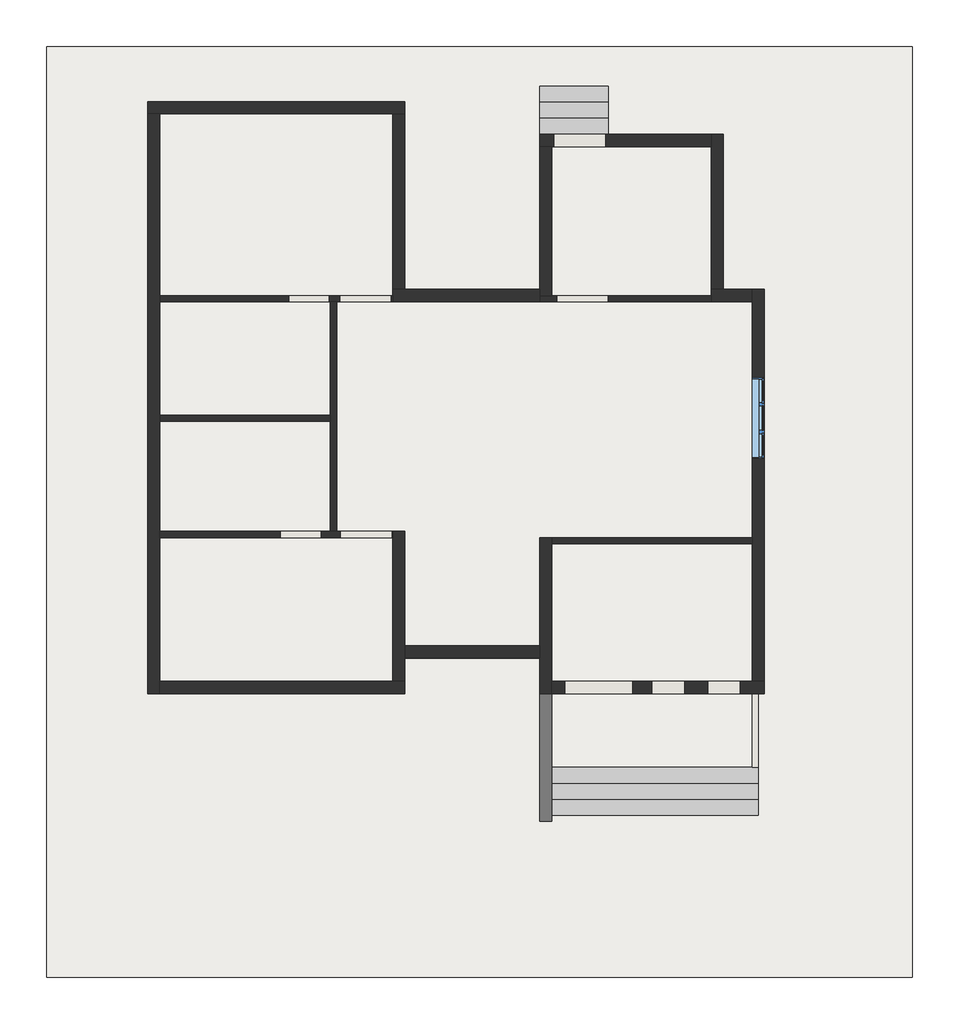
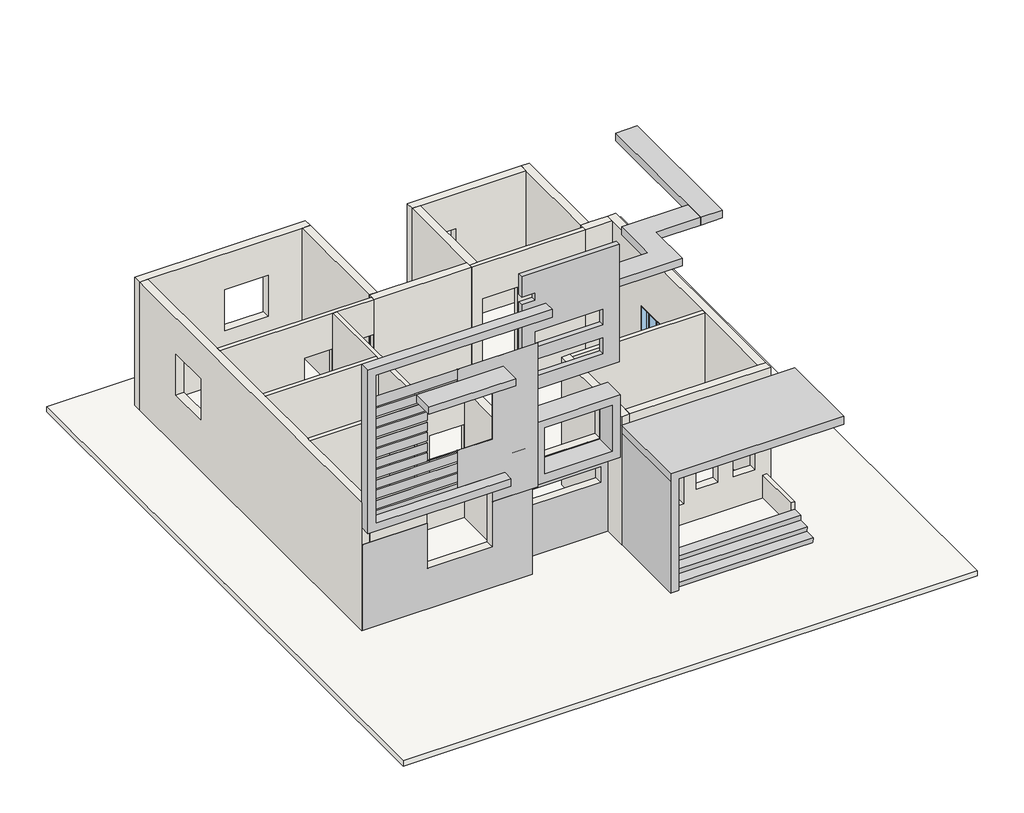
# One storey: 21 walls, 2 stair flights, 1 proxy, 1 slab, 1 window.
"""IFC4 building model written with IfcOpenShell, lengths in millimetres."""

from ifc_helpers import new_model, si_unit, frame, origin, origin_with_axes, place, context, project, spatial, polyline, outline, extrude, faceted_brep, transform, mapped, element, save
from components import generic_models_1_generic_models_1_ca1a1a43, window_casement_triple_middle_transom_5_x4_de6e65d4

model = new_model("IFC4")

# Units and contexts
model_context = context("Model", 3, world=origin())
ifc_project = project(units=[si_unit("LENGTHUNIT", "METRE", prefix="MILLI")], contexts=[model_context])

# Site, building, storey
site = spatial("IfcSite", under=ifc_project)
building = spatial("IfcBuilding", under=site)
storey = spatial("IfcBuildingStorey", under=building, Elevation=0.0)

# Proxy
placement = place(None, origin())
generic_models_1_generic_models_1_shape = generic_models_1_generic_models_1_ca1a1a43(model_context)
element("IfcBuildingElementProxy", 1, Name="Generic Models 1 : Generic Models 1", ObjectType="Generic Models 1 : Generic Models 1", at=placement, inside=storey, context=model_context, shape_type="MappedRepresentation", body=[
    mapped(generic_models_1_generic_models_1_shape, transform((0.0, 0.0, 0.0), x_axis=(1.0, 0.0, 0.0), y_axis=(0.0, 1.0, 0.0), z_axis=(0.0, 0.0, 1.0))),
])

# Slab
element("IfcSlab", 2, ObjectType="site floor", at=placement, inside=storey, context=model_context, shape_type="SweptSolid", body=[
    extrude(outline(polyline([(6700.8181677, 11356.791643), (6700.8181677, -6016.808357), (-9453.5818323, -6016.808357), (-9453.5818323, 11356.791643), (6700.8181677, 11356.791643)])), frame((0.0, 0.0, -152.4), z_axis=(0.0, 0.0, 1.0), x_axis=(1.0, 0.0, 0.0)), (0.0, 0.0, 1.0), 152.4),
])

# Stair flights
element("IfcStairFlight", 3, ObjectType="00 steps", at=placement, inside=storey, context=model_context, shape_type="Brep", body=[
    faceted_brep([(3826.8250448, -2992.8214711, 152.4), (-21.2749552, -2992.8214711, 152.4), (-21.2749552, -2973.7714711, 0.0), (3826.8250448, -2973.7714711, 0.0), (3826.8250448, -2673.7339711, 152.4), (-21.2749552, -2673.7339711, 152.4), (-21.2749552, -2673.7339711, 0.0), (3826.8250448, -2673.7339711, 0.0), (-21.2749552, -2692.7839711, 304.8), (3826.8250448, -2692.7839711, 304.8), (3826.8250448, -2373.7339711, 304.8), (-21.2749552, -2373.7339711, 304.8), (-21.2749552, -2373.7339711, 0.0), (3826.8250448, -2373.7339711, 0.0), (-21.2749552, -2092.7839711, 0.0), (3826.8250448, -2092.7839711, 0.0), (-21.2749552, -2392.7839711, 457.2), (3826.8250448, -2392.7839711, 457.2), (3826.8250448, -2092.7839711, 457.2), (-21.2749552, -2092.7839711, 457.2)], [[[0, 1, 2, 3]], [[1, 0, 4, 5]], [[1, 5, 6, 2]], [[4, 0, 3, 7]], [[8, 9, 10, 11]], [[6, 5, 8, 11, 12]], [[4, 7, 13, 10, 9]], [[5, 4, 9, 8]], [[2, 6, 12, 14, 15, 13, 7, 3]], [[16, 17, 18, 19]], [[12, 11, 16, 19, 14]], [[10, 13, 15, 18, 17]], [[19, 18, 15, 14]], [[11, 10, 17, 16]]]),
])
element("IfcStairFlight", 4, ObjectType="00 steps", at=placement, inside=storey, context=model_context, shape_type="Brep", body=[
    faceted_brep([(-249.8749552, 10618.0535289, 152.4), (1032.8250448, 10618.0535289, 152.4), (1032.8250448, 10599.0035289, 0.0), (-249.8749552, 10599.0035289, 0.0), (-249.8749552, 10298.9660289, 152.4), (1032.8250448, 10298.9660289, 152.4), (1032.8250448, 10298.9660289, 0.0), (-249.8749552, 10298.9660289, 0.0), (1032.8250448, 10318.0160289, 304.8), (-249.8749552, 10318.0160289, 304.8), (-249.8749552, 9998.9660289, 304.8), (1032.8250448, 9998.9660289, 304.8), (1032.8250448, 9998.9660289, 0.0), (-249.8749552, 9998.9660289, 0.0), (1032.8250448, 9718.0160289, 0.0), (-249.8749552, 9718.0160289, 0.0), (1032.8250448, 10018.0160289, 457.2), (-249.8749552, 10018.0160289, 457.2), (-249.8749552, 9718.0160289, 457.2), (1032.8250448, 9718.0160289, 457.2)], [[[0, 1, 2, 3]], [[1, 0, 4, 5]], [[1, 5, 6, 2]], [[4, 0, 3, 7]], [[8, 9, 10, 11]], [[6, 5, 8, 11, 12]], [[4, 7, 13, 10, 9]], [[5, 4, 9, 8]], [[2, 6, 12, 14, 15, 13, 7, 3]], [[16, 17, 18, 19]], [[12, 11, 16, 19, 14]], [[10, 13, 15, 18, 17]], [[19, 18, 15, 14]], [[11, 10, 17, 16]]]),
])

# Walls
element("IfcWall", 5, ObjectType="4.5\" wall", at=placement, inside=storey, context=model_context, shape_type="Brep", body=[
    faceted_brep([(-2993.0749552, 6708.1160289, 0.0), (-7336.4749552, 6708.1160289, 0.0), (-7336.4749552, 6708.1160289, 3810.0), (-2993.0749552, 6708.1160289, 3810.0), (-3018.4749552, 6708.1160289, 609.6), (-3018.4749552, 6708.1160289, 2768.6), (-3983.6749552, 6708.1160289, 2768.6), (-3983.6749552, 6708.1160289, 609.6), (-4936.1749552, 6708.1160289, 609.6), (-4174.1749552, 6708.1160289, 609.6), (-4174.1749552, 6708.1160289, 2743.2), (-4936.1749552, 6708.1160289, 2743.2), (-7336.4749552, 6593.8160289, 0.0), (-4155.1249552, 6593.8160289, 0.0), (-4040.8249552, 6593.8160289, 0.0), (-2993.0749552, 6593.8160289, 0.0), (-2993.0749552, 6593.8160289, 3810.0), (-4040.8249552, 6593.8160289, 3810.0), (-4155.1249552, 6593.8160289, 3810.0), (-7336.4749552, 6593.8160289, 3810.0), (-3018.4749552, 6593.8160289, 2768.6), (-3018.4749552, 6593.8160289, 609.6), (-3983.6749552, 6593.8160289, 609.6), (-3983.6749552, 6593.8160289, 2768.6), (-4936.1749552, 6593.8160289, 609.6), (-4936.1749552, 6593.8160289, 2743.2), (-4174.1749552, 6593.8160289, 2743.2), (-4174.1749552, 6593.8160289, 609.6)], [[[0, 1, 2, 3], [4, 5, 6, 7], [8, 9, 10, 11]], [[12, 13, 14, 15, 16, 17, 18, 19], [20, 21, 22, 23], [24, 25, 26, 27]], [[1, 0, 15, 14, 13, 12]], [[3, 2, 19, 18, 17, 16]], [[0, 3, 16, 15]], [[2, 1, 12, 19]], [[4, 21, 20, 5]], [[5, 20, 23, 6]], [[6, 23, 22, 7]], [[21, 4, 7, 22]], [[9, 8, 24, 27]], [[10, 9, 27, 26]], [[11, 10, 26, 25]], [[8, 11, 25, 24]]]),
])
element("IfcWall", 6, ObjectType="4.5\" wall", at=placement, inside=storey, context=model_context, shape_type="Brep", body=[
    faceted_brep([(-4155.1249552, 6593.8160289, 0.0), (-4155.1249552, 4479.2660289, 0.0), (-4155.1249552, 4364.9660289, 0.0), (-4155.1249552, 2307.5660289, 0.0), (-4155.1249552, 2307.5660289, 3810.0), (-4155.1249552, 4364.9660289, 3810.0), (-4155.1249552, 4479.2660289, 3810.0), (-4155.1249552, 6593.8160289, 3810.0), (-4040.8249552, 6593.8160289, 0.0), (-4040.8249552, 6593.8160289, 3810.0), (-4040.8249552, 2307.5660289, 3810.0), (-4040.8249552, 2307.5660289, 0.0)], [[[0, 1, 2, 3, 4, 5, 6, 7]], [[8, 9, 10, 11]], [[3, 2, 1, 0, 8, 11]], [[7, 6, 5, 4, 10, 9]], [[0, 7, 9, 8]], [[4, 3, 11, 10]]]),
])
element("IfcWall", 7, ObjectType="4.5\" wall", at=placement, inside=storey, context=model_context, shape_type="Brep", body=[
    faceted_brep([(-2993.0749552, 2307.5660289, 0.0), (-4040.8249552, 2307.5660289, 0.0), (-4155.1249552, 2307.5660289, 0.0), (-7336.4749552, 2307.5660289, 0.0), (-7336.4749552, 2307.5660289, 3810.0), (-4155.1249552, 2307.5660289, 3810.0), (-4040.8249552, 2307.5660289, 3810.0), (-2993.0749552, 2307.5660289, 3810.0), (-3005.7749552, 2307.5660289, 609.6), (-3005.7749552, 2307.5660289, 2768.6), (-3970.9749552, 2307.5660289, 2768.6), (-3970.9749552, 2307.5660289, 609.6), (-5088.5749552, 2307.5660289, 609.6), (-4326.5749552, 2307.5660289, 609.6), (-4326.5749552, 2307.5660289, 2743.2), (-5088.5749552, 2307.5660289, 2743.2), (-7336.4749552, 2193.2660289, 0.0), (-2993.0749552, 2193.2660289, 0.0), (-2993.0749552, 2193.2660289, 3810.0), (-7336.4749552, 2193.2660289, 3810.0), (-3005.7749552, 2193.2660289, 2768.6), (-3005.7749552, 2193.2660289, 609.6), (-3970.9749552, 2193.2660289, 609.6), (-3970.9749552, 2193.2660289, 2768.6), (-5088.5749552, 2193.2660289, 609.6), (-5088.5749552, 2193.2660289, 2743.2), (-4326.5749552, 2193.2660289, 2743.2), (-4326.5749552, 2193.2660289, 609.6)], [[[0, 1, 2, 3, 4, 5, 6, 7], [8, 9, 10, 11], [12, 13, 14, 15]], [[16, 17, 18, 19], [20, 21, 22, 23], [24, 25, 26, 27]], [[3, 2, 1, 0, 17, 16]], [[7, 6, 5, 4, 19, 18]], [[4, 3, 16, 19]], [[0, 7, 18, 17]], [[8, 21, 20, 9]], [[9, 20, 23, 10]], [[10, 23, 22, 11]], [[21, 8, 11, 22]], [[13, 12, 24, 27]], [[14, 13, 27, 26]], [[15, 14, 26, 25]], [[12, 15, 25, 24]]]),
])
element("IfcWall", 8, ObjectType="4.5\" wall", at=placement, inside=storey, context=model_context, shape_type="SweptSolid", body=[
    extrude(outline(polyline([(-7336.4749552, 4479.2660289), (-4155.1249552, 4479.2660289), (-4155.1249552, 4364.9660289), (-7336.4749552, 4364.9660289), (-7336.4749552, 4479.2660289)])), origin_with_axes(), (0.0, 0.0, 1.0), 3810.0),
])
element("IfcWall", 9, ObjectType="4.5\" wall", at=placement, inside=storey, context=model_context, shape_type="SweptSolid", body=[
    extrude(outline(polyline([(3712.5250448, 2078.9660289), (-21.2749552, 2078.9660289), (-21.2749552, 2193.2660289), (3712.5250448, 2193.2660289), (3712.5250448, 2078.9660289)])), origin_with_axes(), (0.0, 0.0, 1.0), 3810.0),
])
element("IfcWall", 10, ObjectType="4.5\" wall", at=placement, inside=storey, context=model_context, shape_type="Brep", body=[
    faceted_brep([(2950.5250448, 6708.1160289, 0.0), (-21.2749552, 6708.1160289, 0.0), (-249.8749552, 6708.1160289, 0.0), (-249.8749552, 6708.1160289, 3810.0), (-21.2749552, 6708.1160289, 3810.0), (2950.5250448, 6708.1160289, 3810.0), (67.6250448, 6708.1160289, 2768.6), (67.6250448, 6708.1160289, 609.6), (1032.8250448, 6708.1160289, 609.6), (1032.8250448, 6708.1160289, 2768.6), (-249.8749552, 6593.8160289, 0.0), (2950.5250448, 6593.8160289, 0.0), (2950.5250448, 6593.8160289, 3810.0), (-249.8749552, 6593.8160289, 3810.0), (67.6250448, 6593.8160289, 609.6), (67.6250448, 6593.8160289, 2768.6), (1032.8250448, 6593.8160289, 2768.6), (1032.8250448, 6593.8160289, 609.6)], [[[0, 1, 2, 3, 4, 5], [6, 7, 8, 9]], [[10, 11, 12, 13], [14, 15, 16, 17]], [[2, 1, 0, 11, 10]], [[5, 4, 3, 13, 12]], [[0, 5, 12, 11]], [[3, 2, 10, 13]], [[14, 7, 6, 15]], [[15, 6, 9, 16]], [[16, 9, 8, 17]], [[7, 14, 17, 8]]]),
])
element("IfcWall", 11, ObjectType="4.5\" wall", at=placement, inside=storey, context=model_context, shape_type="SweptSolid", body=[
    extrude(outline(polyline([(3712.5250448, -2092.7839711), (3712.5250448, -734.0839711), (3826.8250448, -734.0839711), (3826.8250448, -2092.7839711), (3712.5250448, -2092.7839711)])), origin_with_axes(), (0.0, 0.0, 1.0), 684.609375),
])
element("IfcWall", 12, ObjectType="9\" wall", at=placement, inside=storey, context=model_context, shape_type="Brep", body=[
    faceted_brep([(-2764.4749552, 10327.6160289, 0.0), (-7565.0749552, 10327.6160289, 0.0), (-7565.0749552, 10327.6160289, 3810.0), (-2764.4749552, 10327.6160289, 3810.0), (-3945.5749552, 10327.6160289, 2743.2), (-5164.7749552, 10327.6160289, 2743.2), (-5164.7749552, 10327.6160289, 1524.0), (-3945.5749552, 10327.6160289, 1524.0), (-2764.4749552, 10099.0160289, 0.0), (-2764.4749552, 10099.0160289, 3810.0), (-2993.0749552, 10099.0160289, 3810.0), (-7336.4749552, 10099.0160289, 3810.0), (-7565.0749552, 10099.0160289, 3810.0), (-7565.0749552, 10099.0160289, 0.0), (-7336.4749552, 10099.0160289, 0.0), (-2993.0749552, 10099.0160289, 0.0), (-3945.5749552, 10099.0160289, 2743.2), (-3945.5749552, 10099.0160289, 1524.0), (-5164.7749552, 10099.0160289, 1524.0), (-5164.7749552, 10099.0160289, 2743.2)], [[[0, 1, 2, 3], [4, 5, 6, 7]], [[8, 9, 10, 11, 12, 13, 14, 15], [16, 17, 18, 19]], [[1, 0, 8, 15, 14, 13]], [[3, 2, 12, 11, 10, 9]], [[2, 1, 13, 12]], [[0, 3, 9, 8]], [[17, 16, 4, 7]], [[18, 17, 7, 6]], [[19, 18, 6, 5]], [[16, 19, 5, 4]]]),
])
element("IfcWall", 13, ObjectType="9\" wall", at=placement, inside=storey, context=model_context, shape_type="Brep", body=[
    faceted_brep([(-7565.0749552, 10099.0160289, 0.0), (-7565.0749552, -721.3839711, 0.0), (-7565.0749552, -721.3839711, 3810.0), (-7565.0749552, 10099.0160289, 3810.0), (-7565.0749552, 8327.3660289, 2743.2), (-7565.0749552, 7108.1660289, 2743.2), (-7565.0749552, 7108.1660289, 1524.0), (-7565.0749552, 8327.3660289, 1524.0), (-7336.4749552, 10099.0160289, 0.0), (-7336.4749552, 10099.0160289, 3810.0), (-7336.4749552, 6708.1160289, 3810.0), (-7336.4749552, 6593.8160289, 3810.0), (-7336.4749552, 4479.2660289, 3810.0), (-7336.4749552, 4364.9660289, 3810.0), (-7336.4749552, 2307.5660289, 3810.0), (-7336.4749552, 2193.2660289, 3810.0), (-7336.4749552, -492.7839711, 3810.0), (-7336.4749552, -721.3839711, 3810.0), (-7336.4749552, -721.3839711, 0.0), (-7336.4749552, -492.7839711, 0.0), (-7336.4749552, 2193.2660289, 0.0), (-7336.4749552, 2307.5660289, 0.0), (-7336.4749552, 4364.9660289, 0.0), (-7336.4749552, 4479.2660289, 0.0), (-7336.4749552, 6593.8160289, 0.0), (-7336.4749552, 6708.1160289, 0.0), (-7336.4749552, 8327.3660289, 2743.2), (-7336.4749552, 8327.3660289, 1524.0), (-7336.4749552, 7108.1660289, 1524.0), (-7336.4749552, 7108.1660289, 2743.2)], [[[0, 1, 2, 3], [4, 5, 6, 7]], [[8, 9, 10, 11, 12, 13, 14, 15, 16, 17, 18, 19, 20, 21, 22, 23, 24, 25], [26, 27, 28, 29]], [[1, 0, 8, 25, 24, 23, 22, 21, 20, 19, 18]], [[3, 2, 17, 16, 15, 14, 13, 12, 11, 10, 9]], [[0, 3, 9, 8]], [[2, 1, 18, 17]], [[27, 26, 4, 7]], [[28, 27, 7, 6]], [[29, 28, 6, 5]], [[26, 29, 5, 4]]]),
])
element("IfcWall", 14, ObjectType="9\" wall", at=placement, inside=storey, context=model_context, shape_type="Brep", body=[
    faceted_brep([(-7336.4749552, -721.3839711, 0.0), (-2764.4749552, -721.3839711, 0.0), (-2764.4749552, -721.3839711, 3810.0), (-7336.4749552, -721.3839711, 3810.0), (-3894.7749552, -721.3839711, 3073.4), (-3894.7749552, -721.3839711, 1219.2), (-5723.5749552, -721.3839711, 1219.2), (-5723.5749552, -721.3839711, 3073.4), (-2764.4749552, -492.7839711, 0.0), (-2993.0749552, -492.7839711, 0.0), (-7336.4749552, -492.7839711, 0.0), (-7336.4749552, -492.7839711, 3810.0), (-2993.0749552, -492.7839711, 3810.0), (-2764.4749552, -492.7839711, 3810.0), (-3894.7749552, -492.7839711, 1219.2), (-3894.7749552, -492.7839711, 3073.4), (-5723.5749552, -492.7839711, 3073.4), (-5723.5749552, -492.7839711, 1219.2)], [[[0, 1, 2, 3], [4, 5, 6, 7]], [[8, 9, 10, 11, 12, 13], [14, 15, 16, 17]], [[1, 0, 10, 9, 8]], [[3, 2, 13, 12, 11]], [[0, 3, 11, 10]], [[2, 1, 8, 13]], [[14, 5, 4, 15]], [[15, 4, 7, 16]], [[16, 7, 6, 17]], [[5, 14, 17, 6]]]),
])
element("IfcWall", 15, ObjectType="9\" wall", at=placement, inside=storey, context=model_context, shape_type="Brep", body=[
    faceted_brep([(-2764.4749552, -492.7839711, 0.0), (-2764.4749552, -54.6339711, 0.0), (-2764.4749552, 173.9660289, 0.0), (-2764.4749552, 2307.5660289, 0.0), (-2764.4749552, 2307.5660289, 3810.0), (-2764.4749552, 173.9660289, 3810.0), (-2764.4749552, -54.6339711, 3810.0), (-2764.4749552, -492.7839711, 3810.0), (-2993.0749552, -492.7839711, 0.0), (-2993.0749552, -492.7839711, 3810.0), (-2993.0749552, 2193.2660289, 3810.0), (-2993.0749552, 2307.5660289, 3810.0), (-2993.0749552, 2307.5660289, 0.0), (-2993.0749552, 2193.2660289, 0.0)], [[[0, 1, 2, 3, 4, 5, 6, 7]], [[8, 9, 10, 11, 12, 13]], [[3, 2, 1, 0, 8, 13, 12]], [[7, 6, 5, 4, 11, 10, 9]], [[0, 7, 9, 8]], [[4, 3, 12, 11]]]),
])
element("IfcWall", 16, ObjectType="9\" wall", at=placement, inside=storey, context=model_context, shape_type="SweptSolid", body=[
    extrude(outline(polyline([(0.0, -2764.4749552), (0.0, -249.8749552), (3810.0, -249.8749552), (3810.0, -478.4749552), (2845.1879698, -478.4749552), (2845.1879698, -2380.0564961), (3810.0, -2380.0564961), (3810.0, -2764.4749552), (0.0, -2764.4749552)]), holes=[polyline([(1524.0, -2593.0249552), (1981.2, -2593.0249552), (1981.2, -459.4249552), (1524.0, -459.4249552), (1524.0, -2593.0249552)])]), frame((0.0, -54.6339711, 0.0), z_axis=(0.0, 1.0, 0.0), x_axis=(0.0, 0.0, 1.0)), (0.0, 0.0, 1.0), 228.6),
])
element("IfcWall", 17, ObjectType="9\" wall", at=placement, inside=storey, context=model_context, shape_type="Brep", body=[
    faceted_brep([(-21.2749552, -721.3839711, 0.0), (-21.2749552, -492.7839711, 0.0), (-21.2749552, 2078.9660289, 0.0), (-21.2749552, 2193.2660289, 0.0), (-21.2749552, 2193.2660289, 3810.0), (-21.2749552, 2078.9660289, 3810.0), (-21.2749552, -492.7839711, 3810.0), (-21.2749552, -721.3839711, 3810.0), (-249.8749552, -721.3839711, 0.0), (-249.8749552, -721.3839711, 3810.0), (-249.8749552, -54.6339711, 3810.0), (-249.8749552, 173.9660289, 3810.0), (-249.8749552, 2193.2660289, 3810.0), (-249.8749552, 2193.2660289, 0.0), (-249.8749552, 173.9660289, 0.0), (-249.8749552, -54.6339711, 0.0)], [[[0, 1, 2, 3, 4, 5, 6, 7]], [[8, 9, 10, 11, 12, 13, 14, 15]], [[3, 2, 1, 0, 8, 15, 14, 13]], [[7, 6, 5, 4, 12, 11, 10, 9]], [[0, 7, 9, 8]], [[4, 3, 13, 12]]]),
])
element("IfcWall", 18, ObjectType="9\" wall", at=placement, inside=storey, context=model_context, shape_type="Brep", body=[
    faceted_brep([(-21.2749552, -721.3839711, 0.0), (3941.1250448, -721.3839711, 0.0), (3941.1250448, -721.3839711, 3810.0), (-21.2749552, -721.3839711, 3810.0), (220.0250448, -721.3839711, 609.6), (220.0250448, -721.3839711, 3073.4), (1490.0250448, -721.3839711, 3073.4), (1490.0250448, -721.3839711, 609.6), (3496.6250448, -721.3839711, 3073.4), (3496.6250448, -721.3839711, 914.4), (2887.0250448, -721.3839711, 914.4), (2887.0250448, -721.3839711, 3073.4), (1845.6250448, -721.3839711, 914.4), (1845.6250448, -721.3839711, 3073.4), (2455.2250448, -721.3839711, 3073.4), (2455.2250448, -721.3839711, 914.4), (3941.1250448, -492.7839711, 0.0), (3712.5250448, -492.7839711, 0.0), (-21.2749552, -492.7839711, 0.0), (-21.2749552, -492.7839711, 3810.0), (3712.5250448, -492.7839711, 3810.0), (3941.1250448, -492.7839711, 3810.0), (220.0250448, -492.7839711, 3073.4), (220.0250448, -492.7839711, 609.6), (1490.0250448, -492.7839711, 609.6), (1490.0250448, -492.7839711, 3073.4), (3496.6250448, -492.7839711, 914.4), (3496.6250448, -492.7839711, 3073.4), (2887.0250448, -492.7839711, 3073.4), (2887.0250448, -492.7839711, 914.4), (1845.6250448, -492.7839711, 3073.4), (1845.6250448, -492.7839711, 914.4), (2455.2250448, -492.7839711, 914.4), (2455.2250448, -492.7839711, 3073.4)], [[[0, 1, 2, 3], [4, 5, 6, 7], [8, 9, 10, 11], [12, 13, 14, 15]], [[16, 17, 18, 19, 20, 21], [22, 23, 24, 25], [26, 27, 28, 29], [30, 31, 32, 33]], [[1, 0, 18, 17, 16]], [[3, 2, 21, 20, 19]], [[0, 3, 19, 18]], [[2, 1, 16, 21]], [[4, 23, 22, 5]], [[5, 22, 25, 6]], [[24, 7, 6, 25]], [[23, 4, 7, 24]], [[26, 9, 8, 27]], [[27, 8, 11, 28]], [[28, 11, 10, 29]], [[9, 26, 29, 10]], [[30, 13, 12, 31]], [[13, 30, 33, 14]], [[14, 33, 32, 15]], [[31, 12, 15, 32]]]),
])
element("IfcWall", 19, ObjectType="9\" wall", at=placement, inside=storey, context=model_context, shape_type="Brep", body=[
    faceted_brep([(3941.1250448, -492.7839711, 0.0), (3941.1250448, 6822.4160289, 0.0), (3941.1250448, 6822.4160289, 3810.0), (3941.1250448, -492.7839711, 3810.0), (3941.1250448, 3660.1160289, 2133.6), (3941.1250448, 5184.1160289, 2133.6), (3941.1250448, 5184.1160289, 914.4), (3941.1250448, 3660.1160289, 914.4), (3712.5250448, -492.7839711, 0.0), (3712.5250448, -492.7839711, 3810.0), (3712.5250448, 2078.9660289, 3810.0), (3712.5250448, 2193.2660289, 3810.0), (3712.5250448, 6593.8160289, 3810.0), (3712.5250448, 6822.4160289, 3810.0), (3712.5250448, 6822.4160289, 0.0), (3712.5250448, 6593.8160289, 0.0), (3712.5250448, 2193.2660289, 0.0), (3712.5250448, 2078.9660289, 0.0), (3712.5250448, 3660.1160289, 2133.6), (3712.5250448, 3660.1160289, 914.4), (3712.5250448, 5184.1160289, 914.4), (3712.5250448, 5184.1160289, 2133.6)], [[[0, 1, 2, 3], [4, 5, 6, 7]], [[8, 9, 10, 11, 12, 13, 14, 15, 16, 17], [18, 19, 20, 21]], [[1, 0, 8, 17, 16, 15, 14]], [[3, 2, 13, 12, 11, 10, 9]], [[0, 3, 9, 8]], [[2, 1, 14, 13]], [[19, 18, 4, 7]], [[20, 19, 7, 6]], [[21, 20, 6, 5]], [[18, 21, 5, 4]]]),
])
element("IfcWall", 20, ObjectType="9\" wall", at=placement, inside=storey, context=model_context, shape_type="Brep", body=[
    faceted_brep([(3712.5250448, 6822.4160289, 0.0), (3179.1250448, 6822.4160289, 0.0), (2950.5250448, 6822.4160289, 0.0), (2950.5250448, 6822.4160289, 3810.0), (3179.1250448, 6822.4160289, 3810.0), (3712.5250448, 6822.4160289, 3810.0), (3712.5250448, 6593.8160289, 0.0), (3712.5250448, 6593.8160289, 3810.0), (2950.5250448, 6593.8160289, 3810.0), (2950.5250448, 6593.8160289, 0.0), (2950.5250448, 6708.1160289, 0.0), (2950.5250448, 6708.1160289, 3810.0)], [[[0, 1, 2, 3, 4, 5]], [[6, 7, 8, 9]], [[2, 1, 0, 6, 9, 10]], [[5, 4, 3, 11, 8, 7]], [[0, 5, 7, 6]], [[3, 2, 10, 9, 8, 11]]]),
])
element("IfcWall", 21, ObjectType="9\" wall", at=placement, inside=storey, context=model_context, shape_type="Brep", body=[
    faceted_brep([(3179.1250448, 6822.4160289, 0.0), (3179.1250448, 9718.0160289, 0.0), (3179.1250448, 9718.0160289, 3810.0), (3179.1250448, 6822.4160289, 3810.0), (2950.5250448, 6822.4160289, 0.0), (2950.5250448, 6822.4160289, 3810.0), (2950.5250448, 9489.4160289, 3810.0), (2950.5250448, 9718.0160289, 3810.0), (2950.5250448, 9718.0160289, 0.0), (2950.5250448, 9489.4160289, 0.0)], [[[0, 1, 2, 3]], [[4, 5, 6, 7, 8, 9]], [[1, 0, 4, 9, 8]], [[3, 2, 7, 6, 5]], [[0, 3, 5, 4]], [[2, 1, 8, 7]]]),
])
element("IfcWall", 22, ObjectType="9\" wall", at=placement, inside=storey, context=model_context, shape_type="Brep", body=[
    faceted_brep([(2950.5250448, 9718.0160289, 0.0), (-249.8749552, 9718.0160289, 0.0), (-249.8749552, 9718.0160289, 3810.0), (2950.5250448, 9718.0160289, 3810.0), (16.8250448, 9718.0160289, 2768.6), (16.8250448, 9718.0160289, 609.6), (982.0250448, 9718.0160289, 609.6), (982.0250448, 9718.0160289, 2768.6), (-249.8749552, 9489.4160289, 0.0), (-21.2749552, 9489.4160289, 0.0), (2950.5250448, 9489.4160289, 0.0), (2950.5250448, 9489.4160289, 3810.0), (-21.2749552, 9489.4160289, 3810.0), (-249.8749552, 9489.4160289, 3810.0), (16.8250448, 9489.4160289, 609.6), (16.8250448, 9489.4160289, 2768.6), (982.0250448, 9489.4160289, 2768.6), (982.0250448, 9489.4160289, 609.6)], [[[0, 1, 2, 3], [4, 5, 6, 7]], [[8, 9, 10, 11, 12, 13], [14, 15, 16, 17]], [[1, 0, 10, 9, 8]], [[3, 2, 13, 12, 11]], [[0, 3, 11, 10]], [[2, 1, 8, 13]], [[14, 5, 4, 15]], [[15, 4, 7, 16]], [[16, 7, 6, 17]], [[5, 14, 17, 6]]]),
])
element("IfcWall", 23, ObjectType="9\" wall", at=placement, inside=storey, context=model_context, shape_type="Brep", body=[
    faceted_brep([(-249.8749552, 9489.4160289, 0.0), (-249.8749552, 6822.4160289, 0.0), (-249.8749552, 6708.1160289, 0.0), (-249.8749552, 6708.1160289, 3810.0), (-249.8749552, 6822.4160289, 3810.0), (-249.8749552, 9489.4160289, 3810.0), (-21.2749552, 9489.4160289, 0.0), (-21.2749552, 9489.4160289, 3810.0), (-21.2749552, 6708.1160289, 3810.0), (-21.2749552, 6708.1160289, 0.0)], [[[0, 1, 2, 3, 4, 5]], [[6, 7, 8, 9]], [[2, 1, 0, 6, 9]], [[5, 4, 3, 8, 7]], [[0, 5, 7, 6]], [[3, 2, 9, 8]]]),
])
element("IfcWall", 24, ObjectType="9\" wall", at=placement, inside=storey, context=model_context, shape_type="Brep", body=[
    faceted_brep([(-249.8749552, 6822.4160289, 0.0), (-2764.4749552, 6822.4160289, 0.0), (-2993.0749552, 6822.4160289, 0.0), (-2993.0749552, 6822.4160289, 3810.0), (-2764.4749552, 6822.4160289, 3810.0), (-249.8749552, 6822.4160289, 3810.0), (-249.8749552, 6593.8160289, 0.0), (-249.8749552, 6593.8160289, 3810.0), (-2993.0749552, 6593.8160289, 3810.0), (-2993.0749552, 6593.8160289, 0.0), (-249.8749552, 6708.1160289, 0.0), (-2993.0749552, 6708.1160289, 0.0), (-2993.0749552, 6708.1160289, 3810.0), (-249.8749552, 6708.1160289, 3810.0)], [[[0, 1, 2, 3, 4, 5]], [[6, 7, 8, 9]], [[2, 1, 0, 10, 6, 9, 11]], [[5, 4, 3, 12, 8, 7, 13]], [[3, 2, 11, 9, 8, 12]], [[0, 5, 13, 7, 6, 10]]]),
])
element("IfcWall", 25, ObjectType="9\" wall", at=placement, inside=storey, context=model_context, shape_type="SweptSolid", body=[
    extrude(outline(polyline([(-2764.4749552, 10099.0160289), (-2764.4749552, 6822.4160289), (-2993.0749552, 6822.4160289), (-2993.0749552, 10099.0160289), (-2764.4749552, 10099.0160289)])), origin_with_axes(), (0.0, 0.0, 1.0), 3810.0),
])

# Window
window_casement_triple_middle_transom_5_x4_shape = window_casement_triple_middle_transom_5_x4_de6e65d4(model_context)
element("IfcWindow", 26, ObjectType="Window-Casement-Triple-Middle-Transom : 5' x4'", at=placement, inside=storey, context=model_context, shape_type="MappedRepresentation", body=[
    mapped(window_casement_triple_middle_transom_5_x4_shape, transform((3826.8250448, 4422.1160289, 0.0), x_axis=(0.0, -1.0, 0.0), y_axis=(1.0, 0.0, 0.0), z_axis=(0.0, 0.0, 1.0))),
])

save(model, "model.ifc")

# Revit data of these elements
# Type "site floor"
#   Assembly Code = "B1010"
#   Function = 0
#   Layers, outside or top first: 0' - 6" "site floor" (function 1)
# Type "4.5\" wall"
#   Assembly Code = "B2010"
#   Layers, outside or top first: 0' - 4 1/2" "Gypsum Wall Board" (function 1)
# Type "9\" wall"
#   Assembly Code = "B2010"
#   Layers, outside or top first: 0' - 9" "Gypsum Wall Board" (function 1)
# Type "Window-Casement-Triple-Middle-Transom : 5' x4'"
#   Type Mark = "26"
#   Fire Rating = "0.5h"
#   Assembly Code = "B2020100"
#   Analytic Construction = "Double glazing - domestic"
#   Window Width = 1' - 8"
#   Window Inset [instance default] = 0' - 0 5/8"
#   Wall Thickness [instance default] = 0' - 6"
#   Visual Light Transmittance = 0.81
#   Transom Height Ratio = 0.3
#   Thermal Resistance (R) = 1.8146 (h·ft²·°F)/BTU
#   Solar Heat Gain Coefficient = 0.76
#   Rough Width = 5' - 0 1/2"
#   Rough Height = 4' - 0 1/2"
#   Heat Transfer Coefficient (U) = 0.5511 BTU/(h·ft²·°F)
#   Height = 4' - 0"
#   Transom Height = 1' - 2.4"
#   Frame Gap 3 [instance default] = 0' - 1 83/128"
#   Frame Gap 2 [instance default] = 0' - 0 5/8"
#   Frame Gap 1 = 0' - 1 51/128"
#   Default Sill Height = 3' - 0"
#   Width = 5' - 0"
#   Frame Material = Metal - Aluminum
#   Glass Panel Material = Glass
#   Wall Closure = (empty or 0)
# Element 1 (IfcBuildingElementProxy, "Generic Models 1 : Generic Models 1")
#   Phase Created = New Construction
#   Materials on its faces: "Door - Frame", "Laminate, Linen, Matte", "Ash colour", "Linen, White"
# Element 2 (IfcSlab, "site floor")
#   Height Offset From Level = 0' - 0"
#   Phase Created = New Construction
#   Materials on its faces: "site floor"
# Element 3 (IfcStairFlight, "00 steps")
#   Phase Created = New Construction
#   Materials on its faces: "Leather - Black", "Concrete, Cast-in-Place gray", "Gypsum Wall Board"
# Element 4 (IfcStairFlight, "00 steps")
#   Phase Created = New Construction
#   Materials on its faces: "Concrete, Cast-in-Place gray"
# Elements 5, 6, 7, 8, 9, 10 (IfcWall, "4.5\" wall")
#   Top Offset = 0' - 0"
#   Base Offset = 0' - 0"
#   wall height = 12' - 6"
#   Phase Created = New Construction
#   Base Constraint = 0.NPC
#   Top Constraint = 2.FIRST FLOOR
#   Materials on its faces: "Gypsum Wall Board"
# Element 11 (IfcWall, "4.5\" wall")
#   Top Offset = 0' - 2 61/64"
#   Base Offset = 0' - 0"
#   wall height = 2' - 2 61/64"
#   Phase Created = New Construction
#   Base Constraint = 0.NPC
#   Top Constraint = 1. GF
#   Materials on its faces: "Gypsum Wall Board"
# Elements 12, 13, 14, 15, 16, 17, 18, 19, 20, 21, 22, 23, 24, 25 (IfcWall, "9\" wall")
#   Top Offset = 0' - 0"
#   Base Offset = 0' - 0"
#   wall height = 12' - 6"
#   Phase Created = New Construction
#   Base Constraint = 0.NPC
#   Top Constraint = 2.FIRST FLOOR
#   Materials on its faces: "Gypsum Wall Board"
# Element 26 (IfcWindow, "Window-Casement-Triple-Middle-Transom : 5' x4'")
#   Mark = "1"
#   Window Inset = 0' - 0 5/8"
#   Frame Gap 3 = 0' - 1 83/128"
#   Frame Gap 2 = 0' - 0 5/8"
#   Phase Created = New Construction
#   Materials on its faces: "Metal - Aluminum", "Glass"
# Materials
#   "site floor": class "Generic", colour RGB 130 144 124, transparency 0, Description = "Gypsum Wall Board", Cost = 0
#   "Gypsum Wall Board": class "Generic", colour RGB 228 228 228, transparency 0, Description = "Gypsum Wall Board", Cost = 0
#   "Metal - Aluminum": class "Metal", colour RGB 247 247 247, transparency 0
#   "Glass": class "Glass", colour RGB 0 128 192, transparency 0.75, Description = "Soda Lime Glass", Cost = 0
#   "Door - Frame": colour RGB 118 70 51, transparency 0, Cost = 0
#   "Laminate, Linen, Matte": class "Plastic", colour RGB 198 189 176, transparency 0, Description = "Plastic Laminate - Linen, Matte", Cost = 0
#   "Ash colour": class "Generic", colour RGB 94 94 94, transparency 0, Cost = 0
#   "Linen, White": class "Textile", colour RGB 206 206 206, transparency 0, Description = "Linen, white", Cost = 0
#   "Leather - Black": class "Generic", colour RGB 40 40 40, transparency 0, Cost = 0
#   "Concrete, Cast-in-Place gray": class "Concrete", colour RGB 192 192 192, transparency 0, Description = "Cast-in-place concrete", Cost = 0
# Room at (-5285.505, 8440.945) mm, phase "New Construction", upper offset 10' - 0", lower offset 0' - 0"
#   Number = "1"
#   Name = "BEDROOM"
# Room at (1483.76, 8001.465) mm, phase "New Construction", upper offset 10' - 0", lower offset 0' - 0"
#   Number = "2"
#   Name = "KITCHEN"
# Room at (0, 4513.348) mm, phase "New Construction", upper offset 10' - 0", lower offset 0' - 0"
#   Number = "3"
#   Name = "DINING"
# Room at (-5767.113, 5596.719) mm, phase "New Construction", upper offset 10' - 0", lower offset 0' - 0"
#   Number = "4"
#   Name = "TOILET"
# Room at (-5634.839, 3365.18) mm, phase "New Construction", upper offset 10' - 0", lower offset 0' - 0"
#   Number = "5"
#   Name = "TOILET"
# Room at (-5139.114, 984.274) mm, phase "New Construction", upper offset 10' - 0", lower offset 0' - 0"
#   Number = "6"
#   Name = "M-BEDROOM"
# Room at (-1547.908, 1188.756) mm, phase "New Construction", upper offset 10' - 0", lower offset 0' - 0"
#   Number = "7"
#   Name = "STAIR"
# Room at (1828.8, 984.274) mm, phase "New Construction", upper offset 10' - 0", lower offset 0' - 0"
#   Number = "8"
#   Name = "LIVING"
